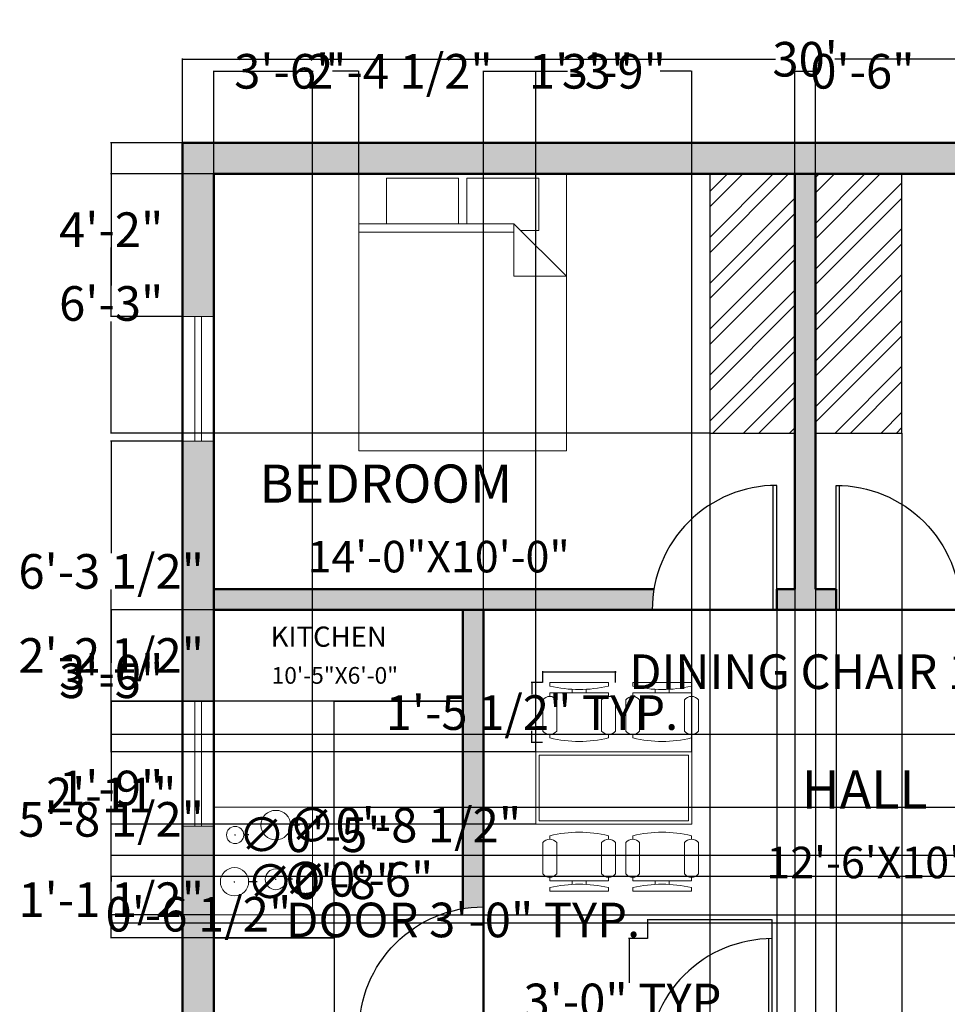
# Model space of a CAD drawing. Units: inches. Extents: x 168 to 640, y -211 to 244.
# Tile 2 of 3: x 168 to 436, y -40 to 244. Entities that reach past the tile are written whole.
import ezdxf

# ---------------------------------------------------------------- set-up
doc = ezdxf.new("R2010")
doc.units = ezdxf.units.IN
doc.header["$MEASUREMENT"] = 0
for name, color, linetype, lineweight in [('A-ANNO-DIMS', 2, 'Continuous', 18), ('A-AREA-IDEN', 7, 'Continuous', 25), ('A-DOOR', 4, 'Continuous', 25), ('A-EQPM', 9, 'Continuous', 18), ('A-FLOR-CASE', 8, 'Continuous', 25), ('A-FLOR-CASE-PATT', 8, 'Continuous', 13), ('A-FURN', 8, 'Continuous', 18), ('A-GLAZ', 4, 'Continuous', 18), ('A-WALL', 7, 'Continuous', 50)]:
    doc.layers.add(name, color=color, linetype=linetype, lineweight=lineweight)
doc.layers.add('A-WALL-PATT', color=251, linetype='Continuous', lineweight=13, true_color=0x636466)
doc.styles.get("Standard").update_dxf_attribs({"font": 'arial.ttf'})
doc.dimstyles.get("Standard").update_dxf_attribs({"dimtxt": 10, "dimasz": 0.18, "dimexe": 0.18, "dimexo": 0.0625, "dimgap": 0.09, "dimtad": 0, "dimtih": 1, "dimtoh": 1, "dimdec": 0, "dimzin": 0, "dimdsep": 46, "dimlunit": 3, "dimtxsty": 'Standard', "dimcen": 0.09, "dimadec": 0, "dimazin": 0, "dimtfac": 1, "dimtdec": 0, "dimtofl": 0, "dimtmove": 0, "dimatfit": 3, "dimfxl": 1, "dimtolj": 1, "dimtzin": 0, "dimarcsym": 0})

# ---------------------------------------------------------------- blocks, each defined once
blk = doc.blocks.new('*D2')
at = {"layer": 'A-ANNO-DIMS', "color": 0, "lineweight": -2, "transparency": 16777216}
for p, q in [((214.63, 208.86), (214.63, 233.12)), ((214.81, 232.94), (386.06, 232.94)), ((574.45, 232.94), (403.21, 232.94)), ((574.63, 208.86), (574.63, 233.12))]:
    blk.add_line(p, q, dxfattribs=at)
at = {"layer": 'A-ANNO-DIMS', "color": 0, "transparency": 16777216}
for points in [[(214.81, 232.97), (214.81, 232.91), (214.63, 232.94)], [(574.45, 232.97), (574.45, 232.91), (574.63, 232.94)]]:
    blk.add_solid(points, dxfattribs=at)
at = {"layer": 'Defpoints', "color": 0, "transparency": 16777216}
for p in [(214.63, 232.94), (214.63, 208.8), (574.63, 208.8)]:
    blk.add_point(p, dxfattribs=at)
at = {"layer": 'A-ANNO-DIMS', "color": 0, "transparency": 16777216, "insert": (394.63, 232.94), "char_height": 10, "attachment_point": 5}
blk.add_mtext("\\A1;30'", dxfattribs=at)
blk = doc.blocks.new('Bed - Queen')
for p, q in [((0, -80.00003), (0, 0)), ((0, 0), (59.99999, 0)), ((59.99999, 0), (59.99999, -80.00003)), ((7.99999, -1.2), (28.79998, -1.2)), ((7.99999, -14.4), (7.99999, -1.2)), ((28.79998, -1.2), (28.79998, -14.4)), ((31.19999, -1.2), (51.99999, -1.2)), ((31.19999, -14.4), (31.19999, -1.2)), ((51.99999, -1.2), (51.99999, -16.4)), ((0, -14.4), (44.8, -14.4)), ((44.8, -16.8), (0, -16.8)), ((59.99999, -29.6), (44.8, -14.4)), ((44.8, -14.4), (44.8, -29.6)), ((51.99999, -16.4), (46.79936, -16.4)), ((44.8, -29.6), (59.99999, -29.6)), ((59.99999, -80.00003), (0, -80.00003))]:
    blk.add_line(p, q)
blk = doc.blocks.new('Chair - Desk')
for p, q in [((-8.5, 0), (-8.5, -1)), ((-8.5, 0), (8.5, 0)), ((8.5, 0), (8.5, -1)), ((-2, -3), (-2, -1.9355)), ((2, -1.9576), (2, -3)), ((-10.5, -5), (-10.5, -14)), ((-8.5, -3), (-8.5, -4)), ((-8.5, -3), (8.5, -3)), ((-6.5, -14), (-6.5, -5)), ((6.5, -5), (6.5, -14)), ((8.5, -3), (8.5, -4)), ((10.5, -14), (10.5, -5)), ((-8.5, -15), (-8.5, -16)), ((8.5, -15), (8.5, -16))]:
    blk.add_line(p, q)
for centre, radius, start, end in [((0, 34.625), 36.625, 256.5803, 283.4197), ((-8.5, -6.5), 2.5, 36.8699, 143.1301), ((8.5, -6.5), 2.5, 36.8699, 143.1301), ((-8.5, -12.5), 2.5, 216.8699, 323.1301), ((8.5, -12.5), 2.5, 216.8699, 323.1301), ((0, 19.625), 36.625, 256.5803, 283.4197)]:
    blk.add_arc(centre, radius, start, end)
blk = doc.blocks.new('DOOR-SWING-36IN')
for p, q in [((0, 36), (0, 0)), ((1, 36), (1, 0))]:
    blk.add_line(p, q)
blk.add_arc((0, 36), 36, 270, 0)
blk = doc.blocks.new('WIN-36IN-WALL9')
at = {"ltscale": 0.25}
for p, q in [((0, 36), (9, 36)), ((3.5, 36), (3.5, 0)), ((5.5, 36), (5.5, 0)), ((9, 0), (0, 0))]:
    blk.add_line(p, q, dxfattribs=at)
blk = doc.blocks.new('*D11')
at = {"layer": 'A-ANNO-DIMS', "color": 0, "lineweight": -2, "ltscale": 0.25, "transparency": 16777216}
for p, q in [((349.12, -15.8), (348.94, -15.8)), ((349.12, -21.14), (349.12, -15.62)), ((384.94, -15.8), (349.3, -15.8)), ((385.12, -21.14), (385.12, -15.62))]:
    blk.add_line(p, q, dxfattribs=at)
at = {"layer": 'A-ANNO-DIMS', "color": 0, "ltscale": 0.25, "transparency": 16777216}
for points in [[(349.3, -15.77), (349.3, -15.83), (349.12, -15.8)], [(384.94, -15.77), (384.94, -15.83), (385.12, -15.8)]]:
    blk.add_solid(points, dxfattribs=at)
at = {"layer": 'Defpoints', "color": 0, "ltscale": 0.25, "transparency": 16777216}
for p in [(349.12, -15.8), (349.12, -21.2), (385.12, -21.2)]:
    blk.add_point(p, dxfattribs=at)
at = {"layer": 'A-ANNO-DIMS', "color": 0, "ltscale": 0.25, "transparency": 16777216, "insert": (295.73, -15.8), "char_height": 10, "attachment_point": 5}
blk.add_mtext('\\A1;DOOR 3\'-0" TYP.', dxfattribs=at)
blk = doc.blocks.new('*D12')
at = {"layer": 'A-ANNO-DIMS', "color": 0, "lineweight": -2, "ltscale": 0.25, "transparency": 16777216}
for p, q in [((349.06, -21.2), (343.54, -21.2)), ((343.72, -21.38), (343.72, -34)), ((343.72, -57.02), (343.72, -44.4)), ((349.06, -57.2), (343.54, -57.2))]:
    blk.add_line(p, q, dxfattribs=at)
at = {"layer": 'A-ANNO-DIMS', "color": 0, "ltscale": 0.25, "transparency": 16777216}
for points in [[(343.69, -21.38), (343.75, -21.38), (343.72, -21.2)], [(343.69, -57.02), (343.75, -57.02), (343.72, -57.2)]]:
    blk.add_solid(points, dxfattribs=at)
at = {"layer": 'Defpoints', "color": 0, "ltscale": 0.25, "transparency": 16777216}
for p in [(349.12, -21.2), (343.72, -57.2), (349.12, -57.2)]:
    blk.add_point(p, dxfattribs=at)
at = {"layer": 'A-ANNO-DIMS', "color": 0, "ltscale": 0.25, "transparency": 16777216, "insert": (343.72, -39.2), "char_height": 10, "attachment_point": 5}
blk.add_mtext('\\A1;3\'-0" TYP.', dxfattribs=at)
blk = doc.blocks.new('*D15')
at = {"layer": 'A-ANNO-DIMS', "color": 0, "lineweight": -2, "ltscale": 0.25, "transparency": 16777216}
for p, q in [((318.79, 52.86), (318.79, 56.13)), ((318.97, 55.95), (339.61, 55.95)), ((339.79, 52.86), (339.79, 56.13)), ((339.79, 55.95), (339.97, 55.95))]:
    blk.add_line(p, q, dxfattribs=at)
at = {"layer": 'A-ANNO-DIMS', "color": 0, "ltscale": 0.25, "transparency": 16777216}
for points in [[(318.97, 55.98), (318.97, 55.92), (318.79, 55.95)], [(339.61, 55.98), (339.61, 55.92), (339.79, 55.95)]]:
    blk.add_solid(points, dxfattribs=at)
at = {"layer": 'Defpoints', "color": 0, "ltscale": 0.25, "transparency": 16777216}
for p in [(339.79, 55.95), (318.79, 52.8), (339.79, 52.8)]:
    blk.add_point(p, dxfattribs=at)
at = {"layer": 'A-ANNO-DIMS', "color": 0, "ltscale": 0.25, "transparency": 16777216, "insert": (420.35, 55.95), "char_height": 10, "attachment_point": 5}
blk.add_mtext('\\A1;DINING CHAIR 1\'-9" TYP.', dxfattribs=at)
blk = doc.blocks.new('*D16')
at = {"layer": 'A-ANNO-DIMS', "color": 0, "lineweight": -2, "ltscale": 0.25, "transparency": 16777216}
for p, q in [((318.73, 52.8), (315.46, 52.8)), ((315.64, 52.62), (315.64, 49.39)), ((315.64, 35.65), (315.64, 38.87)), ((318.73, 35.47), (315.46, 35.47))]:
    blk.add_line(p, q, dxfattribs=at)
at = {"layer": 'A-ANNO-DIMS', "color": 0, "ltscale": 0.25, "transparency": 16777216}
for points in [[(315.61, 52.62), (315.67, 52.62), (315.64, 52.8)], [(315.61, 35.65), (315.67, 35.65), (315.64, 35.47)]]:
    blk.add_solid(points, dxfattribs=at)
at = {"layer": 'Defpoints', "color": 0, "ltscale": 0.25, "transparency": 16777216}
for p in [(315.64, 52.8), (318.79, 52.8), (318.79, 35.47)]:
    blk.add_point(p, dxfattribs=at)
at = {"layer": 'A-ANNO-DIMS', "color": 0, "ltscale": 0.25, "transparency": 16777216, "insert": (315.64, 44.13), "char_height": 10, "attachment_point": 5}
blk.add_mtext('\\A1;1\'-5 1/2" TYP.', dxfattribs=at)
blk = doc.blocks.new('*D21')
at = {"layer": 'A-ANNO-DIMS', "color": 0, "lineweight": -2, "ltscale": 0.25, "transparency": 16777216}
for p, q in [((214.57, 208.8), (193.8, 208.8)), ((193.98, 208.62), (193.98, 188.79)), ((193.98, 158.75), (193.98, 178.57)), ((214.57, 158.57), (193.8, 158.57))]:
    blk.add_line(p, q, dxfattribs=at)
at = {"layer": 'A-ANNO-DIMS', "color": 0, "ltscale": 0.25, "transparency": 16777216}
for points in [[(193.95, 208.62), (194.01, 208.62), (193.98, 208.8)], [(193.95, 158.75), (194.01, 158.75), (193.98, 158.57)]]:
    blk.add_solid(points, dxfattribs=at)
at = {"layer": 'Defpoints', "color": 0, "ltscale": 0.25, "transparency": 16777216}
for p in [(214.63, 208.8), (193.98, 158.57), (214.63, 158.57)]:
    blk.add_point(p, dxfattribs=at)
at = {"layer": 'A-ANNO-DIMS', "color": 0, "ltscale": 0.25, "transparency": 16777216, "insert": (193.98, 183.68), "char_height": 10, "attachment_point": 5}
blk.add_mtext('\\A1;4\'-2"', dxfattribs=at)
blk = doc.blocks.new('*D22')
at = {"layer": 'A-ANNO-DIMS', "color": 0, "lineweight": -2, "ltscale": 0.25, "transparency": 16777216}
for p, q in [((214.57, 122.57), (193.8, 122.57)), ((193.98, 122.39), (193.98, 90.2)), ((193.98, 47.48), (193.98, 79.67)), ((214.57, 47.3), (193.8, 47.3))]:
    blk.add_line(p, q, dxfattribs=at)
at = {"layer": 'A-ANNO-DIMS', "color": 0, "ltscale": 0.25, "transparency": 16777216}
for points in [[(193.95, 122.39), (194.01, 122.39), (193.98, 122.57)], [(193.95, 47.48), (194.01, 47.48), (193.98, 47.3)]]:
    blk.add_solid(points, dxfattribs=at)
at = {"layer": 'Defpoints', "color": 0, "ltscale": 0.25, "transparency": 16777216}
for p in [(214.63, 122.57), (193.98, 47.3), (214.63, 47.3)]:
    blk.add_point(p, dxfattribs=at)
at = {"layer": 'A-ANNO-DIMS', "color": 0, "ltscale": 0.25, "transparency": 16777216, "insert": (193.98, 84.93), "char_height": 10, "attachment_point": 5}
blk.add_mtext('\\A1;6\'-3 1/2"', dxfattribs=at)
blk = doc.blocks.new('*D31')
at = {"layer": 'A-ANNO-DIMS', "color": 0, "lineweight": -2, "ltscale": 0.25, "transparency": 16777216}
for p, q in [((391.63, 199.86), (391.63, 229.63)), ((391.81, 229.45), (397.45, 229.45)), ((397.63, 199.86), (397.63, 229.63)), ((397.63, 229.45), (397.81, 229.45))]:
    blk.add_line(p, q, dxfattribs=at)
at = {"layer": 'A-ANNO-DIMS', "color": 0, "ltscale": 0.25, "transparency": 16777216}
for points in [[(391.81, 229.48), (391.81, 229.42), (391.63, 229.45)], [(397.45, 229.48), (397.45, 229.42), (397.63, 229.45)]]:
    blk.add_solid(points, dxfattribs=at)
at = {"layer": 'Defpoints', "color": 0, "ltscale": 0.25, "transparency": 16777216}
for p in [(397.63, 229.45), (391.63, 199.8), (397.63, 199.8)]:
    blk.add_point(p, dxfattribs=at)
at = {"layer": 'A-ANNO-DIMS', "color": 0, "ltscale": 0.25, "transparency": 16777216, "insert": (411.2, 229.45), "char_height": 10, "attachment_point": 5}
blk.add_mtext('\\A1;0\'-6"', dxfattribs=at)
blk = doc.blocks.new('*D33')
at = {"layer": 'A-ANNO-DIMS', "color": 0, "lineweight": -2, "ltscale": 0.25, "transparency": 16777216}
for p, q in [((565.57, 73.8), (193.8, 73.8)), ((193.98, 73.62), (193.98, 61)), ((193.98, 37.98), (193.98, 50.6)), ((565.57, 37.8), (193.8, 37.8))]:
    blk.add_line(p, q, dxfattribs=at)
at = {"layer": 'A-ANNO-DIMS', "color": 0, "ltscale": 0.25, "transparency": 16777216}
for points in [[(193.95, 73.62), (194.01, 73.62), (193.98, 73.8)], [(193.95, 37.98), (194.01, 37.98), (193.98, 37.8)]]:
    blk.add_solid(points, dxfattribs=at)
at = {"layer": 'Defpoints', "color": 0, "ltscale": 0.25, "transparency": 16777216}
for p in [(193.98, 73.8), (565.63, 73.8), (565.63, 37.8)]:
    blk.add_point(p, dxfattribs=at)
at = {"layer": 'A-ANNO-DIMS', "color": 0, "ltscale": 0.25, "transparency": 16777216, "insert": (193.98, 55.8), "char_height": 10, "attachment_point": 5}
blk.add_mtext('\\A1;3\'-0"', dxfattribs=at)
blk = doc.blocks.new('*D34')
at = {"layer": 'A-ANNO-DIMS', "color": 0, "lineweight": -2, "ltscale": 0.25, "transparency": 16777216}
for p, q in [((451.57, 37.8), (193.8, 37.8)), ((193.98, 37.62), (193.98, 25.41)), ((193.98, 2.98), (193.98, 15.19)), ((451.57, 2.8), (193.8, 2.8))]:
    blk.add_line(p, q, dxfattribs=at)
at = {"layer": 'A-ANNO-DIMS', "color": 0, "ltscale": 0.25, "transparency": 16777216}
for points in [[(193.95, 37.62), (194.01, 37.62), (193.98, 37.8)], [(193.95, 2.98), (194.01, 2.98), (193.98, 2.8)]]:
    blk.add_solid(points, dxfattribs=at)
at = {"layer": 'Defpoints', "color": 0, "ltscale": 0.25, "transparency": 16777216}
for p in [(193.98, 37.8), (451.63, 37.8), (451.63, 2.8)]:
    blk.add_point(p, dxfattribs=at)
at = {"layer": 'A-ANNO-DIMS', "color": 0, "ltscale": 0.25, "transparency": 16777216, "insert": (193.98, 20.3), "char_height": 10, "attachment_point": 5}
blk.add_mtext('\\A1;2\'-11"', dxfattribs=at)
blk = doc.blocks.new('*D35')
at = {"layer": 'A-ANNO-DIMS', "color": 0, "lineweight": -2, "ltscale": 0.25, "transparency": 16777216}
for p, q in [((386.42, 73.74), (386.42, -196.03)), ((403.56, 73.74), (403.56, -196.03)), ((386.6, -195.85), (403.38, -195.85)), ((403.56, -195.85), (403.74, -195.85))]:
    blk.add_line(p, q, dxfattribs=at)
at = {"layer": 'A-ANNO-DIMS', "color": 0, "ltscale": 0.25, "transparency": 16777216}
for points in [[(386.6, -195.82), (386.6, -195.88), (386.42, -195.85)], [(403.38, -195.82), (403.38, -195.88), (403.56, -195.85)]]:
    blk.add_solid(points, dxfattribs=at)
at = {"layer": 'Defpoints', "color": 0, "ltscale": 0.25, "transparency": 16777216}
for p in [(386.42, 73.8), (403.56, 73.8), (403.56, -195.85)]:
    blk.add_point(p, dxfattribs=at)
at = {"layer": 'A-ANNO-DIMS', "color": 0, "ltscale": 0.25, "transparency": 16777216, "insert": (416.65, -195.85), "char_height": 10, "attachment_point": 5}
blk.add_mtext('\\A1;1\'-5"', dxfattribs=at)
blk = doc.blocks.new('*D36')
at = {"layer": 'A-ANNO-DIMS', "color": 0, "lineweight": -2, "ltscale": 0.25, "transparency": 16777216}
for p, q in [((386.42, 79.74), (386.42, -196.03)), ((391.63, 79.74), (391.63, -196.03)), ((386.42, -195.85), (386.24, -195.85)), ((391.45, -195.85), (386.6, -195.85))]:
    blk.add_line(p, q, dxfattribs=at)
at = {"layer": 'A-ANNO-DIMS', "color": 0, "ltscale": 0.25, "transparency": 16777216}
for points in [[(386.6, -195.82), (386.6, -195.88), (386.42, -195.85)], [(391.45, -195.82), (391.45, -195.88), (391.63, -195.85)]]:
    blk.add_solid(points, dxfattribs=at)
at = {"layer": 'Defpoints', "color": 0, "ltscale": 0.25, "transparency": 16777216}
for p in [(386.42, 79.8), (391.63, 79.8), (386.42, -195.85)]:
    blk.add_point(p, dxfattribs=at)
at = {"layer": 'A-ANNO-DIMS', "color": 0, "ltscale": 0.25, "transparency": 16777216, "insert": (372.86, -195.85), "char_height": 10, "attachment_point": 5}
blk.add_mtext('\\A1;0\'-5"', dxfattribs=at)
blk = doc.blocks.new('*D45')
at = {"layer": 'A-ANNO-DIMS', "color": 0, "lineweight": -2, "ltscale": 0.25, "transparency": 16777216}
for p, q in [((223.63, -20.98), (223.63, -196.03)), ((258.47, -20.98), (258.47, -196.03)), ((223.45, -195.85), (223.27, -195.85)), ((258.65, -195.85), (258.83, -195.85))]:
    blk.add_line(p, q, dxfattribs=at)
at = {"layer": 'A-ANNO-DIMS', "color": 0, "ltscale": 0.25, "transparency": 16777216}
for points in [[(223.45, -195.82), (223.45, -195.88), (223.63, -195.85)], [(258.65, -195.82), (258.65, -195.88), (258.47, -195.85)]]:
    blk.add_solid(points, dxfattribs=at)
at = {"layer": 'Defpoints', "color": 0, "ltscale": 0.25, "transparency": 16777216}
for p in [(223.63, -20.92), (258.47, -20.92), (258.47, -195.85)]:
    blk.add_point(p, dxfattribs=at)
at = {"layer": 'A-ANNO-DIMS', "color": 0, "ltscale": 0.25, "transparency": 16777216, "insert": (241.05, -195.85), "char_height": 10, "attachment_point": 5}
blk.add_mtext('\\A1;2\'-11"', dxfattribs=at)
blk = doc.blocks.new('*D46')
at = {"layer": 'A-ANNO-DIMS', "color": 0, "lineweight": -2, "ltscale": 0.25, "transparency": 16777216}
for p, q in [((258.41, 47.47), (193.8, 47.47)), ((193.98, 47.29), (193.98, 18.53)), ((193.98, -20.74), (193.98, 8.01)), ((258.41, -20.92), (193.8, -20.92))]:
    blk.add_line(p, q, dxfattribs=at)
at = {"layer": 'A-ANNO-DIMS', "color": 0, "ltscale": 0.25, "transparency": 16777216}
for points in [[(193.95, 47.29), (194.01, 47.29), (193.98, 47.47)], [(193.95, -20.74), (194.01, -20.74), (193.98, -20.92)]]:
    blk.add_solid(points, dxfattribs=at)
at = {"layer": 'Defpoints', "color": 0, "ltscale": 0.25, "transparency": 16777216}
for p in [(193.98, 47.47), (258.47, 47.47), (258.47, -20.92)]:
    blk.add_point(p, dxfattribs=at)
at = {"layer": 'A-ANNO-DIMS', "color": 0, "ltscale": 0.25, "transparency": 16777216, "insert": (193.98, 13.27), "char_height": 10, "attachment_point": 5}
blk.add_mtext('\\A1;5\'-8 1/2"', dxfattribs=at)
blk = doc.blocks.new('*D47')
at = {"layer": 'A-ANNO-DIMS', "color": 0, "lineweight": -2, "ltscale": 0.25, "transparency": 16777216}
for p, q in [((295.57, 73.8), (193.8, 73.8)), ((193.98, 73.62), (193.98, 65.89)), ((193.98, 47.65), (193.98, 55.37)), ((295.57, 47.47), (193.8, 47.47))]:
    blk.add_line(p, q, dxfattribs=at)
at = {"layer": 'A-ANNO-DIMS', "color": 0, "ltscale": 0.25, "transparency": 16777216}
for points in [[(193.95, 73.62), (194.01, 73.62), (193.98, 73.8)], [(193.95, 47.65), (194.01, 47.65), (193.98, 47.47)]]:
    blk.add_solid(points, dxfattribs=at)
at = {"layer": 'Defpoints', "color": 0, "ltscale": 0.25, "transparency": 16777216}
for p in [(193.98, 73.8), (295.63, 73.8), (295.63, 47.47)]:
    blk.add_point(p, dxfattribs=at)
at = {"layer": 'A-ANNO-DIMS', "color": 0, "ltscale": 0.25, "transparency": 16777216, "insert": (193.98, 60.63), "char_height": 10, "attachment_point": 5}
blk.add_mtext('\\A1;2\'-2 1/2"', dxfattribs=at)
blk = doc.blocks.new('*D48')
at = {"layer": 'A-ANNO-DIMS', "color": 0, "lineweight": -2, "ltscale": 0.25, "transparency": 16777216}
for p, q in [((223.63, 16.86), (223.63, 229.63)), ((223.81, 229.45), (251.99, 229.45)), ((252.17, 16.86), (252.17, 229.63)), ((252.17, 229.45), (252.35, 229.45))]:
    blk.add_line(p, q, dxfattribs=at)
at = {"layer": 'A-ANNO-DIMS', "color": 0, "ltscale": 0.25, "transparency": 16777216}
for points in [[(223.81, 229.48), (223.81, 229.42), (223.63, 229.45)], [(251.99, 229.48), (251.99, 229.42), (252.17, 229.45)]]:
    blk.add_solid(points, dxfattribs=at)
at = {"layer": 'Defpoints', "color": 0, "ltscale": 0.25, "transparency": 16777216}
for p in [(252.17, 229.45), (223.63, 16.8), (252.17, 16.8)]:
    blk.add_point(p, dxfattribs=at)
at = {"layer": 'A-ANNO-DIMS', "color": 0, "ltscale": 0.25, "transparency": 16777216, "insert": (277.47, 229.45), "char_height": 10, "attachment_point": 5}
blk.add_mtext('\\A1;2\'-4 1/2"', dxfattribs=at)
blk = doc.blocks.new('*D49')
at = {"layer": 'A-ANNO-DIMS', "color": 0, "lineweight": -2, "ltscale": 0.25, "transparency": 16777216}
for p, q in [((252.23, 16.8), (595.46, 16.8)), ((595.28, 16.62), (595.28, 6.35)), ((595.28, -14.14), (595.28, -3.87)), ((252.23, -14.32), (595.46, -14.32))]:
    blk.add_line(p, q, dxfattribs=at)
at = {"layer": 'A-ANNO-DIMS', "color": 0, "ltscale": 0.25, "transparency": 16777216}
for points in [[(595.25, 16.62), (595.31, 16.62), (595.28, 16.8)], [(595.25, -14.14), (595.31, -14.14), (595.28, -14.32)]]:
    blk.add_solid(points, dxfattribs=at)
at = {"layer": 'Defpoints', "color": 0, "ltscale": 0.25, "transparency": 16777216}
for p in [(252.17, 16.8), (595.28, 16.8), (252.17, -14.32)]:
    blk.add_point(p, dxfattribs=at)
at = {"layer": 'A-ANNO-DIMS', "color": 0, "ltscale": 0.25, "transparency": 16777216, "insert": (595.28, 1.24), "char_height": 10, "attachment_point": 5}
blk.add_mtext('\\A1;2\'-7"', dxfattribs=at)
blk = doc.blocks.new('*D50')
at = {"layer": 'A-ANNO-DIMS', "color": 0, "lineweight": -2, "ltscale": 0.25, "transparency": 16777216}
for p, q in [((193.98, -14.32), (193.98, -14.14)), ((193.98, -14.14), (194.16, -14.14)), ((223.57, -14.32), (193.8, -14.32)), ((193.98, -20.74), (193.98, -14.5)), ((223.57, -20.92), (193.8, -20.92))]:
    blk.add_line(p, q, dxfattribs=at)
at = {"layer": 'A-ANNO-DIMS', "color": 0, "ltscale": 0.25, "transparency": 16777216}
for points in [[(193.95, -14.5), (194.01, -14.5), (193.98, -14.32)], [(193.95, -20.74), (194.01, -20.74), (193.98, -20.92)]]:
    blk.add_solid(points, dxfattribs=at)
at = {"layer": 'Defpoints', "color": 0, "ltscale": 0.25, "transparency": 16777216}
for p in [(193.98, -14.32), (223.63, -14.32), (223.63, -20.92)]:
    blk.add_point(p, dxfattribs=at)
at = {"layer": 'A-ANNO-DIMS', "color": 0, "ltscale": 0.25, "transparency": 16777216, "insert": (219.2, -14.14), "char_height": 10, "attachment_point": 5}
blk.add_mtext('\\A1;0\'-6 1/2"', dxfattribs=at)
blk = doc.blocks.new('*D51')
at = {"layer": 'A-ANNO-DIMS', "color": 0, "lineweight": -2, "ltscale": 0.25, "transparency": 16777216}
for p, q in [((316.76, 32.89), (316.76, 229.63)), ((316.94, 229.45), (325.95, 229.45)), ((361.72, 229.45), (352.71, 229.45)), ((361.9, 32.89), (361.9, 229.63))]:
    blk.add_line(p, q, dxfattribs=at)
at = {"layer": 'A-ANNO-DIMS', "color": 0, "ltscale": 0.25, "transparency": 16777216}
for points in [[(316.94, 229.48), (316.94, 229.42), (316.76, 229.45)], [(361.72, 229.48), (361.72, 229.42), (361.9, 229.45)]]:
    blk.add_solid(points, dxfattribs=at)
at = {"layer": 'Defpoints', "color": 0, "ltscale": 0.25, "transparency": 16777216}
for p in [(361.9, 229.45), (316.76, 32.83), (361.9, 32.83)]:
    blk.add_point(p, dxfattribs=at)
at = {"layer": 'A-ANNO-DIMS', "color": 0, "ltscale": 0.25, "transparency": 16777216, "insert": (339.33, 229.45), "char_height": 10, "attachment_point": 5}
blk.add_mtext('\\A1;3\'-9"', dxfattribs=at)
blk = doc.blocks.new('*D52')
at = {"layer": 'A-ANNO-DIMS', "color": 0, "lineweight": -2, "ltscale": 0.25, "transparency": 16777216}
for p, q in [((316.7, 32.83), (193.8, 32.83)), ((193.98, 32.65), (193.98, 27.53)), ((193.98, 12.02), (193.98, 17.14)), ((316.7, 11.84), (193.8, 11.84))]:
    blk.add_line(p, q, dxfattribs=at)
at = {"layer": 'A-ANNO-DIMS', "color": 0, "ltscale": 0.25, "transparency": 16777216}
for points in [[(193.95, 32.65), (194.01, 32.65), (193.98, 32.83)], [(193.95, 12.02), (194.01, 12.02), (193.98, 11.84)]]:
    blk.add_solid(points, dxfattribs=at)
at = {"layer": 'Defpoints', "color": 0, "ltscale": 0.25, "transparency": 16777216}
for p in [(193.98, 32.83), (316.76, 32.83), (316.76, 11.84)]:
    blk.add_point(p, dxfattribs=at)
at = {"layer": 'A-ANNO-DIMS', "color": 0, "ltscale": 0.25, "transparency": 16777216, "insert": (193.98, 22.33), "char_height": 10, "attachment_point": 5}
blk.add_mtext('\\A1;1\'-9"', dxfattribs=at)
blk = doc.blocks.new('*D53')
at = {"layer": 'A-ANNO-DIMS', "color": 0, "lineweight": -2, "ltscale": 0.25, "transparency": 16777216}
for p, q in [((367.04, 124.86), (367.04, -196.03)), ((391.63, 124.86), (391.63, -196.03)), ((367.22, -195.85), (391.45, -195.85)), ((391.63, -195.85), (391.81, -195.85))]:
    blk.add_line(p, q, dxfattribs=at)
at = {"layer": 'A-ANNO-DIMS', "color": 0, "ltscale": 0.25, "transparency": 16777216}
for points in [[(367.22, -195.82), (367.22, -195.88), (367.04, -195.85)], [(391.45, -195.82), (391.45, -195.88), (391.63, -195.85)]]:
    blk.add_solid(points, dxfattribs=at)
at = {"layer": 'Defpoints', "color": 0, "ltscale": 0.25, "transparency": 16777216}
for p in [(367.04, 124.92), (391.63, 124.92), (391.63, -195.85)]:
    blk.add_point(p, dxfattribs=at)
at = {"layer": 'A-ANNO-DIMS', "color": 0, "ltscale": 0.25, "transparency": 16777216, "insert": (416.93, -195.85), "char_height": 10, "attachment_point": 5}
blk.add_mtext('\\A1;2\'-0 1/2"', dxfattribs=at)
blk = doc.blocks.new('*D54')
at = {"layer": 'A-ANNO-DIMS', "color": 0, "lineweight": -2, "ltscale": 0.25, "transparency": 16777216}
for p, q in [((366.98, 199.8), (193.8, 199.8)), ((193.98, 199.62), (193.98, 167.56)), ((193.98, 125.1), (193.98, 157.16)), ((366.98, 124.92), (193.8, 124.92))]:
    blk.add_line(p, q, dxfattribs=at)
at = {"layer": 'A-ANNO-DIMS', "color": 0, "ltscale": 0.25, "transparency": 16777216}
for points in [[(193.95, 199.62), (194.01, 199.62), (193.98, 199.8)], [(193.95, 125.1), (194.01, 125.1), (193.98, 124.92)]]:
    blk.add_solid(points, dxfattribs=at)
at = {"layer": 'Defpoints', "color": 0, "ltscale": 0.25, "transparency": 16777216}
for p in [(193.98, 199.8), (367.04, 199.8), (367.04, 124.92)]:
    blk.add_point(p, dxfattribs=at)
at = {"layer": 'A-ANNO-DIMS', "color": 0, "ltscale": 0.25, "transparency": 16777216, "insert": (193.98, 162.36), "char_height": 10, "attachment_point": 5}
blk.add_mtext('\\A1;6\'-3"', dxfattribs=at)
blk = doc.blocks.new('*D55')
at = {"layer": 'A-ANNO-DIMS', "color": 0, "lineweight": -2, "ltscale": 0.25, "transparency": 16777216}
for p, q in [((397.63, 124.86), (397.63, -196.03)), ((422.63, 124.86), (422.63, -196.03)), ((397.81, -195.85), (422.45, -195.85)), ((422.63, -195.85), (422.81, -195.85))]:
    blk.add_line(p, q, dxfattribs=at)
at = {"layer": 'A-ANNO-DIMS', "color": 0, "ltscale": 0.25, "transparency": 16777216}
for points in [[(397.81, -195.82), (397.81, -195.88), (397.63, -195.85)], [(422.45, -195.82), (422.45, -195.88), (422.63, -195.85)]]:
    blk.add_solid(points, dxfattribs=at)
at = {"layer": 'Defpoints', "color": 0, "ltscale": 0.25, "transparency": 16777216}
for p in [(397.63, 124.92), (422.63, 124.92), (422.63, -195.85)]:
    blk.add_point(p, dxfattribs=at)
at = {"layer": 'A-ANNO-DIMS', "color": 0, "ltscale": 0.25, "transparency": 16777216, "insert": (436.28, -195.85), "char_height": 10, "attachment_point": 5}
blk.add_mtext('\\A1;2\'-1"', dxfattribs=at)
blk = doc.blocks.new('*D56')
at = {"layer": 'A-ANNO-DIMS', "color": 0, "lineweight": -2, "ltscale": 0.25, "transparency": 16777216}
for p, q in [((223.63, 199.86), (223.63, 229.63)), ((223.81, 229.45), (231.25, 229.45)), ((265.43, 229.45), (258, 229.45)), ((265.61, 199.86), (265.61, 229.63))]:
    blk.add_line(p, q, dxfattribs=at)
at = {"layer": 'A-ANNO-DIMS', "color": 0, "ltscale": 0.25, "transparency": 16777216}
for points in [[(223.81, 229.48), (223.81, 229.42), (223.63, 229.45)], [(265.43, 229.48), (265.43, 229.42), (265.61, 229.45)]]:
    blk.add_solid(points, dxfattribs=at)
at = {"layer": 'Defpoints', "color": 0, "ltscale": 0.25, "transparency": 16777216}
for p in [(265.61, 229.45), (223.63, 199.8), (265.61, 199.8)]:
    blk.add_point(p, dxfattribs=at)
at = {"layer": 'A-ANNO-DIMS', "color": 0, "ltscale": 0.25, "transparency": 16777216, "insert": (244.62, 229.45), "char_height": 10, "attachment_point": 5}
blk.add_mtext('\\A1;3\'-6"', dxfattribs=at)
blk = doc.blocks.new('*D60')
at = {"layer": 'A-ANNO-DIMS', "color": 0, "lineweight": -2, "ltscale": 0.25, "transparency": 16777216}
for p, q in [((301.63, 73.86), (301.63, 229.63)), ((301.81, 229.45), (316.58, 229.45)), ((316.76, 32.89), (316.76, 229.63)), ((316.76, 229.45), (316.94, 229.45))]:
    blk.add_line(p, q, dxfattribs=at)
at = {"layer": 'A-ANNO-DIMS', "color": 0, "ltscale": 0.25, "transparency": 16777216}
for points in [[(301.81, 229.48), (301.81, 229.42), (301.63, 229.45)], [(316.58, 229.48), (316.58, 229.42), (316.76, 229.45)]]:
    blk.add_solid(points, dxfattribs=at)
at = {"layer": 'Defpoints', "color": 0, "ltscale": 0.25, "transparency": 16777216}
for p in [(316.76, 229.45), (301.63, 73.8), (316.76, 32.83)]:
    blk.add_point(p, dxfattribs=at)
at = {"layer": 'A-ANNO-DIMS', "color": 0, "ltscale": 0.25, "transparency": 16777216, "insert": (329.85, 229.45), "char_height": 10, "attachment_point": 5}
blk.add_mtext('\\A1;1\'-3"', dxfattribs=at)
blk = doc.blocks.new('*D61')
at = {"layer": 'A-ANNO-DIMS', "color": 0, "lineweight": -2, "ltscale": 0.25, "transparency": 16777216}
for p, q in [((301.57, 73.8), (193.8, 73.8)), ((193.98, 73.62), (193.98, 58.51)), ((193.98, 33.01), (193.98, 48.12)), ((316.7, 32.83), (193.8, 32.83))]:
    blk.add_line(p, q, dxfattribs=at)
at = {"layer": 'A-ANNO-DIMS', "color": 0, "ltscale": 0.25, "transparency": 16777216}
for points in [[(193.95, 73.62), (194.01, 73.62), (193.98, 73.8)], [(193.95, 33.01), (194.01, 33.01), (193.98, 32.83)]]:
    blk.add_solid(points, dxfattribs=at)
at = {"layer": 'Defpoints', "color": 0, "ltscale": 0.25, "transparency": 16777216}
for p in [(301.63, 73.8), (193.98, 32.83), (316.76, 32.83)]:
    blk.add_point(p, dxfattribs=at)
at = {"layer": 'A-ANNO-DIMS', "color": 0, "ltscale": 0.25, "transparency": 16777216, "insert": (193.98, 53.32), "char_height": 10, "attachment_point": 5}
blk.add_mtext('\\A1;3\'-5"', dxfattribs=at)
blk = doc.blocks.new('*D62')
at = {"layer": 'A-ANNO-DIMS', "color": 0, "lineweight": -2, "ltscale": 0.25, "transparency": 16777216}
for p, q in [((565.57, -3.2), (193.8, -3.2)), ((193.98, -3.38), (193.98, -4.69)), ((565.57, -16.7), (193.8, -16.7)), ((193.98, -16.52), (193.98, -15.21))]:
    blk.add_line(p, q, dxfattribs=at)
at = {"layer": 'A-ANNO-DIMS', "color": 0, "ltscale": 0.25, "transparency": 16777216}
for points in [[(193.95, -3.38), (194.01, -3.38), (193.98, -3.2)], [(193.95, -16.52), (194.01, -16.52), (193.98, -16.7)]]:
    blk.add_solid(points, dxfattribs=at)
at = {"layer": 'Defpoints', "color": 0, "ltscale": 0.25, "transparency": 16777216}
for p in [(565.63, -3.2), (193.98, -16.7), (565.63, -16.7)]:
    blk.add_point(p, dxfattribs=at)
at = {"layer": 'A-ANNO-DIMS', "color": 0, "ltscale": 0.25, "transparency": 16777216, "insert": (193.98, -9.95), "char_height": 10, "attachment_point": 5}
blk.add_mtext('\\A1;1\'-1 1/2"', dxfattribs=at)
blk = doc.blocks.new('*D63')
at = {"layer": 'A-ANNO-DIMS', "color": 0, "lineweight": -2, "ltscale": 0.25, "transparency": 16777216}
for p, q in [((241.47, 11.61), (241.65, 11.61)), ((241.56, 11.52), (241.56, 11.7)), ((248.4, 11.61), (246.01, 11.61))]:
    blk.add_line(p, q, dxfattribs=at)
at = {"layer": 'A-ANNO-DIMS', "color": 0, "ltscale": 0.25, "transparency": 16777216}
blk.add_solid([(246.01, 11.64), (246.01, 11.58), (245.83, 11.61)], dxfattribs=at)
at = {"layer": 'Defpoints', "color": 0, "ltscale": 0.25, "transparency": 16777216}
for p in [(237.29, 11.61), (245.83, 11.61)]:
    blk.add_point(p, dxfattribs=at)
at = {"layer": 'A-ANNO-DIMS', "color": 0, "ltscale": 0.25, "transparency": 16777216, "insert": (278.87, 11.61), "char_height": 10, "attachment_point": 5}
blk.add_mtext('\\A1;∅0\'-8 1/2"', dxfattribs=at)
blk = doc.blocks.new('*D64')
at = {"layer": 'A-ANNO-DIMS', "color": 0, "lineweight": -2, "ltscale": 0.25, "transparency": 16777216}
for p, q in [((229.54, -4.76), (229.72, -4.76)), ((229.63, -4.85), (229.63, -4.67)), ((236.18, -4.76), (233.9, -4.76))]:
    blk.add_line(p, q, dxfattribs=at)
at = {"layer": 'A-ANNO-DIMS', "color": 0, "ltscale": 0.25, "transparency": 16777216}
blk.add_solid([(233.9, -4.73), (233.9, -4.79), (233.72, -4.76)], dxfattribs=at)
at = {"layer": 'Defpoints', "color": 0, "ltscale": 0.25, "transparency": 16777216}
for p in [(225.54, -4.76), (233.72, -4.76)]:
    blk.add_point(p, dxfattribs=at)
at = {"layer": 'A-ANNO-DIMS', "color": 0, "ltscale": 0.25, "transparency": 16777216, "insert": (255, -4.76), "char_height": 10, "attachment_point": 5}
blk.add_mtext('\\A1;∅0\'-8"', dxfattribs=at)
blk = doc.blocks.new('*D65')
at = {"layer": 'A-ANNO-DIMS', "color": 0, "lineweight": -2, "ltscale": 0.25, "transparency": 16777216}
for p, q in [((229.72, 8.76), (229.9, 8.76)), ((229.81, 8.67), (229.81, 8.85)), ((233.79, 8.82), (232.48, 8.8))]:
    blk.add_line(p, q, dxfattribs=at)
at = {"layer": 'A-ANNO-DIMS', "color": 0, "ltscale": 0.25, "transparency": 16777216}
blk.add_solid([(232.48, 8.83), (232.48, 8.77), (232.3, 8.8)], dxfattribs=at)
at = {"layer": 'Defpoints', "color": 0, "ltscale": 0.25, "transparency": 16777216}
for p in [(227.32, 8.72), (232.3, 8.8)]:
    blk.add_point(p, dxfattribs=at)
at = {"layer": 'A-ANNO-DIMS', "color": 0, "ltscale": 0.25, "transparency": 16777216, "insert": (252.61, 8.82), "char_height": 10, "attachment_point": 5}
blk.add_mtext('\\A1;∅0\'-5"', dxfattribs=at)
blk = doc.blocks.new('*D66')
at = {"layer": 'A-ANNO-DIMS', "color": 0, "lineweight": -2, "ltscale": 0.25, "transparency": 16777216}
for p, q in [((241.47, -4.05), (241.65, -4.05)), ((241.56, -4.14), (241.56, -3.96)), ((246.4, -4.05), (244.77, -4.05))]:
    blk.add_line(p, q, dxfattribs=at)
at = {"layer": 'A-ANNO-DIMS', "color": 0, "ltscale": 0.25, "transparency": 16777216}
blk.add_solid([(244.77, -4.02), (244.77, -4.08), (244.59, -4.05)], dxfattribs=at)
at = {"layer": 'Defpoints', "color": 0, "ltscale": 0.25, "transparency": 16777216}
for p in [(238.54, -4.05), (244.59, -4.05)]:
    blk.add_point(p, dxfattribs=at)
at = {"layer": 'A-ANNO-DIMS', "color": 0, "ltscale": 0.25, "transparency": 16777216, "insert": (265.22, -4.05), "char_height": 10, "attachment_point": 5}
blk.add_mtext('\\A1;∅0\'-6"', dxfattribs=at)

msp = doc.modelspace()

# ---------------------------------------------------------------- hatches: boundary and pattern name
at = {"layer": 'A-FLOR-CASE-PATT', "ltscale": 0.25}
h = msp.add_hatch(dxfattribs=at)
h.set_pattern_fill('ANSI32', color=256, scale=25)
h.paths.add_polyline_path([(391.63, 199.8), (367.04, 199.8), (367.04, 124.92), (391.63, 124.92)])
h.paths.add_polyline_path([(422.63, 199.8), (397.63, 199.8), (397.63, 124.92), (422.63, 124.92)])
at = {"layer": 'A-WALL-PATT', "ltscale": 0.25}
h = msp.add_hatch(color=256, dxfattribs=at)
h.dxf.hatch_style = 1
h.paths.add_polyline_path([(223.63, 11.3), (214.63, 11.3), (214.63, -175.2), (574.63, -175.2), (574.63, -137.43), (565.63, -137.43), (565.63, -157.06), (565.63, -166.2), (223.63, -166.2)])
h.paths.add_polyline_path([(349.62, -51.2), (301.63, -51.2), (223.63, -51.2), (223.63, -57.2), (301.63, -57.2), (349.12, -57.2, -0.041886)], flags=17)
h.paths.add_polyline_path([(301.63, -48.03), (295.63, -48.03), (295.63, -51.2), (301.63, -51.2)], flags=17)
h.paths.add_polyline_path([(403.8, -51.2), (385.12, -51.2), (385.12, -57.2), (403.8, -57.2)], flags=17)
h.paths.add_polyline_path([(397.63, -57.2), (390.63, -57.2), (390.63, -166.2), (397.63, -166.2)], flags=17)
h.paths.add_polyline_path([(301.63, 73.8), (295.63, 73.8), (295.63, -12.53, -0.041886), (301.63, -12.03)])
h.paths.add_polyline_path([(223.63, 122.57), (214.63, 122.57), (214.63, 47.3), (223.63, 47.3), (223.63, 73.8)])
h.paths.add_polyline_path([(350.92, 79.8), (223.63, 79.8), (223.63, 73.8), (350.42, 73.8, -0.041886)])
h.paths.add_polyline_path([(574.63, 208.8), (214.63, 208.8), (214.63, 158.57), (223.63, 158.57), (223.63, 199.8), (565.63, 199.8), (565.63, 158.57), (574.63, 158.57)])
h.paths.add_polyline_path([(397.63, 199.8), (391.63, 199.8), (391.63, 79.8), (386.42, 79.8), (386.42, 73.8), (391.63, 73.8), (403.56, 73.8), (403.56, 79.8), (397.63, 79.8)])
h.paths.add_polyline_path([(565.63, 79.8), (439.06, 79.8, -0.041886), (439.56, 73.8), (565.63, 73.8)])
h.paths.add_polyline_path([(574.63, 122.57), (565.63, 122.57), (565.63, 79.8), (565.63, 52.8), (574.63, 52.8)])
h.paths.add_polyline_path([(574.63, 16.8), (565.63, 16.8), (565.63, -15.33), (574.63, -15.33)])
h.paths.add_polyline_path([(574.63, -39.29), (570.13, -39.29), (565.63, -39.29), (565.63, -51.2), (565.63, -101.43), (574.63, -101.43)], flags=17)
h.paths.add_polyline_path([(565.63, -51.2), (439.8, -51.2, -0.041886), (439.3, -57.2), (565.63, -57.2)], flags=17)

# ---------------------------------------------------------------- linework, layer by layer
at = {"layer": 'A-EQPM', "ltscale": 0.25}
for p, q in [((223.63, 16.8), (252.17, 16.8)), ((252.17, 16.8), (252.17, -14.32)), ((252.17, -14.32), (223.63, -14.32))]:
    msp.add_line(p, q, dxfattribs=at)
for centre, radius in [((241.56, 11.61), 4.27), ((229.81, 8.76), 2.49), ((229.63, -4.76), 4.09), ((241.56, -4.05), 3.02)]:
    msp.add_circle(centre, radius, dxfattribs=at)
at = {"layer": 'A-FLOR-CASE', "ltscale": 0.25}
for p, q in [((367.04, 199.8), (367.04, 124.92)), ((422.63, 124.92), (422.63, 199.8)), ((367.04, 124.92), (391.63, 124.92)), ((397.63, 124.92), (422.63, 124.92)), ((258.47, -20.92), (258.47, 47.47)), ((258.47, 47.47), (295.63, 47.47)), ((223.63, -20.92), (258.47, -20.92))]:
    msp.add_line(p, q, dxfattribs=at)
at = {"layer": 'A-FURN', "ltscale": 0.25}
for points in [[(316.76, 32.83), (361.9, 32.83), (361.9, 11.84), (316.76, 11.84)], [(317.76, 31.83), (360.9, 31.83), (360.9, 12.84), (317.76, 12.84)]]:
    msp.add_lwpolyline(points, close=True, dxfattribs=at)
at = {"layer": 'A-GLAZ', "ltscale": 0.25}
msp.add_line((219.13, 122.57), (223.63, 122.57), dxfattribs=at)
at = {"layer": 'A-WALL'}
for p, q in [((214.63, 208.8), (574.63, 208.8)), ((214.63, 208.8), (214.63, -175.2)), ((223.63, 199.8), (565.63, 199.8)), ((223.63, 199.8), (223.63, -166.2)), ((223.63, 79.8), (223.63, 199.8)), ((391.63, 79.8), (391.63, 199.8)), ((391.63, 199.8), (391.63, 79.8)), ((397.63, 79.8), (397.63, 199.8)), ((350.92, 79.8), (223.63, 79.8)), ((391.63, 79.8), (386.42, 79.8)), ((386.42, 79.8), (386.42, 73.8)), ((403.56, 79.8), (397.63, 79.8)), ((403.56, 79.8), (403.56, 73.8)), ((391.63, 73.8), (223.63, 73.8)), ((223.63, 73.8), (223.63, -51.2)), ((295.63, -12.53), (295.63, 73.8)), ((301.63, -51.2), (301.63, 73.8)), ((565.63, 73.8), (391.63, 73.8))]:
    msp.add_line(p, q, dxfattribs=at)

# ---------------------------------------------------------------- block references
at = {"layer": 'A-DOOR', "rotation": 180}
for p in [(386.42, 109.8), (385.12, -21.2)]:
    msp.add_blockref('DOOR-SWING-36IN', p, dxfattribs=at)
at = {"layer": 'A-DOOR', "extrusion": (0, 0, -1), "zscale": -1}
for p, rotation in [((-403.56, 109.8), 180), ((-265.63, -48.03), 90.00000000000007)]:
    msp.add_blockref('DOOR-SWING-36IN', p, dxfattribs=dict(at, rotation=rotation))
at = {"layer": 'A-FURN', "ltscale": 0.25}
for name, p in [('Bed - Queen', (265.61, 199.8)), ('Chair - Desk', (329.29, 52.8)), ('Chair - Desk', (353.28, 52.8))]:
    msp.add_blockref(name, p, dxfattribs=at)
at = {"layer": 'A-FURN', "ltscale": 0.25, "xscale": -1, "rotation": 180}
for p in [(329.29, -7.46), (353.28, -7.46)]:
    msp.add_blockref('Chair - Desk', p, dxfattribs=at)
at = {"layer": 'A-GLAZ'}
for p in [(214.63, 122.57), (214.63, 11.3)]:
    msp.add_blockref('WIN-36IN-WALL9', p, dxfattribs=at)

# ---------------------------------------------------------------- texts
at = {"layer": 'A-AREA-IDEN', "ltscale": 0.25}
for s, height, p in [('BEDROOM', 11.012, (236.82, 104.8)), ('14\'-0"X10\'-0"', 9.1115, (250.74, 84.64)), ('KITCHEN  ', 5.839, (240.1, 63.15)), ('10\'-5"X6\'-0"', 4.8311, (240.36, 52.46)), ('HALL  ', 11.012, (393.66, 16.41)), ('12\'-6\'X10\'-5"', 9.1115, (383.42, -3.75))]:
    msp.add_text(s, height=height, dxfattribs=at).set_placement(p)

# ---------------------------------------------------------------- dimensions: what is measured, and where the dimension line sits
at = {"layer": 'A-ANNO-DIMS', "ltscale": 0.25}
for base, p1, p2, picture, middle in [((252.17, 229.45), (223.63, 16.8), (252.17, 16.8), '*D48', (277.47, 229.45)), ((265.61, 229.45), (223.63, 199.8), (265.61, 199.8), '*D56', (244.62, 229.45)), ((316.76, 229.45), (301.63, 73.8), (316.76, 32.83), '*D60', (329.85, 229.45)), ((361.9, 229.45), (316.76, 32.83), (361.9, 32.83), '*D51', (339.33, 229.45)), ((397.63, 229.45), (391.63, 199.8), (397.63, 199.8), '*D31', (411.2, 229.45)), ((391.63, -195.85), (367.04, 124.92), (391.63, 124.92), '*D53', (416.93, -195.85)), ((422.63, -195.85), (397.63, 124.92), (422.63, 124.92), '*D55', (436.28, -195.85)), ((386.42, -195.85), (391.63, 79.8), (386.42, 79.8), '*D36', (372.86, -195.85)), ((403.56, -195.85), (386.42, 73.8), (403.56, 73.8), '*D35', (416.65, -195.85)), ((258.47, -195.85), (223.63, -20.92), (258.47, -20.92), '*D45', (241.05, -195.85))]:
    dim = msp.add_linear_dim(base=base, p1=p1, p2=p2, dimstyle='Standard', override={"dimdec": 1, "dimlfac": 1, "dimrnd": 0, "dimzin": 1, "dimdsep": 46, "dimlunit": 4, "dimfrac": 2}, dxfattribs=at)
    dim.commit()
    dim.dimension.update_dxf_attribs({"geometry": picture, "text_midpoint": middle})
at = {"layer": 'A-ANNO-DIMS'}
dim = msp.add_linear_dim(base=(214.63, 232.94), p1=(574.63, 208.8), p2=(214.63, 208.8), dimstyle='Standard', override={"dimclrd": 0, "dimclre": 0, "dimclrt": 0}, dxfattribs=at)
dim.commit()
dim.dimension.update_dxf_attribs({"geometry": '*D2', "text_midpoint": (394.63, 232.94)})
at = {"layer": 'A-ANNO-DIMS', "ltscale": 0.25}
for base, p1, p2, picture, middle in [((193.98, 158.57), (214.63, 208.8), (214.63, 158.57), '*D21', (193.98, 183.68)), ((193.98, 199.8), (367.04, 124.92), (367.04, 199.8), '*D54', (193.98, 162.36)), ((193.98, 47.3), (214.63, 122.57), (214.63, 47.3), '*D22', (193.98, 84.93)), ((193.98, 73.8), (295.63, 47.47), (295.63, 73.8), '*D47', (193.98, 60.63)), ((193.98, 73.8), (565.63, 37.8), (565.63, 73.8), '*D33', (193.98, 55.8)), ((193.98, 32.83), (301.63, 73.8), (316.76, 32.83), '*D61', (193.98, 53.32)), ((193.98, 47.47), (258.47, -20.92), (258.47, 47.47), '*D46', (193.98, 13.27)), ((193.98, 37.8), (451.63, 2.8), (451.63, 37.8), '*D34', (193.98, 20.3)), ((193.98, 32.83), (316.76, 11.84), (316.76, 32.83), '*D52', (193.98, 22.33)), ((595.28, 16.8), (252.17, -14.32), (252.17, 16.8), '*D49', (595.28, 1.24)), ((193.98, -16.7), (565.63, -3.2), (565.63, -16.7), '*D62', (193.98, -9.95)), ((193.98, -14.32), (223.63, -20.92), (223.63, -14.32), '*D50', (219.2, -14.14))]:
    dim = msp.add_linear_dim(base=base, p1=p1, p2=p2, angle=90, dimstyle='Standard', override={"dimdec": 1, "dimlfac": 1, "dimrnd": 0, "dimzin": 1, "dimdsep": 46, "dimlunit": 4, "dimfrac": 2}, dxfattribs=at)
    dim.commit()
    dim.dimension.update_dxf_attribs({"geometry": picture, "text_midpoint": middle})
dim = msp.add_linear_dim(base=(339.79, 55.95), p1=(318.79, 52.8), p2=(339.79, 52.8), text='DINING CHAIR <> TYP.', dimstyle='Standard', override={"dimdec": 1, "dimlfac": 1, "dimrnd": 0, "dimzin": 1, "dimdsep": 46, "dimlunit": 4, "dimfrac": 2}, dxfattribs=at)
dim.commit()
dim.dimension.update_dxf_attribs({"geometry": '*D15', "text_midpoint": (420.35, 55.95)})
for base, p1, p2, angle, text, picture, middle in [((315.64, 52.8), (318.79, 35.47), (318.79, 52.8), 90, '<> TYP.', '*D16', (315.64, 44.13)), ((349.12, -15.8), (385.12, -21.2), (349.12, -21.2), 180, 'DOOR <> TYP.', '*D11', (295.73, -15.8)), ((343.72, -57.2), (349.12, -21.2), (349.12, -57.2), 270, '<> TYP.', '*D12', (343.72, -39.2))]:
    dim = msp.add_linear_dim(base=base, p1=p1, p2=p2, angle=angle, text=text, dimstyle='Standard', override={"dimdec": 1, "dimlfac": 1, "dimrnd": 0, "dimzin": 1, "dimdsep": 46, "dimlunit": 4, "dimfrac": 2}, dxfattribs=at)
    dim.commit()
    dim.dimension.update_dxf_attribs({"geometry": picture, "text_midpoint": middle})
for p1, p2, picture, middle in [((237.29, 11.61), (245.83, 11.61), '*D63', (248.4, 11.61)), ((227.32, 8.72), (232.3, 8.8), '*D65', (233.79, 8.82)), ((225.54, -4.76), (233.72, -4.76), '*D64', (236.18, -4.76)), ((238.5391, -4.05), (244.5886, -4.05), '*D66', (246.4035, -4.05))]:
    dim = msp.add_diameter_dim_2p(p1=p1, p2=p2, dimstyle='Standard', override={"dimdec": 1, "dimlfac": 1, "dimrnd": 0, "dimzin": 1, "dimdsep": 46, "dimlunit": 4, "dimfrac": 2}, dxfattribs=at)
    dim.commit()
    dim.dimension.update_dxf_attribs({"geometry": picture, "text_midpoint": middle, "dimtype": 163})

doc.saveas('drawing.dxf')
